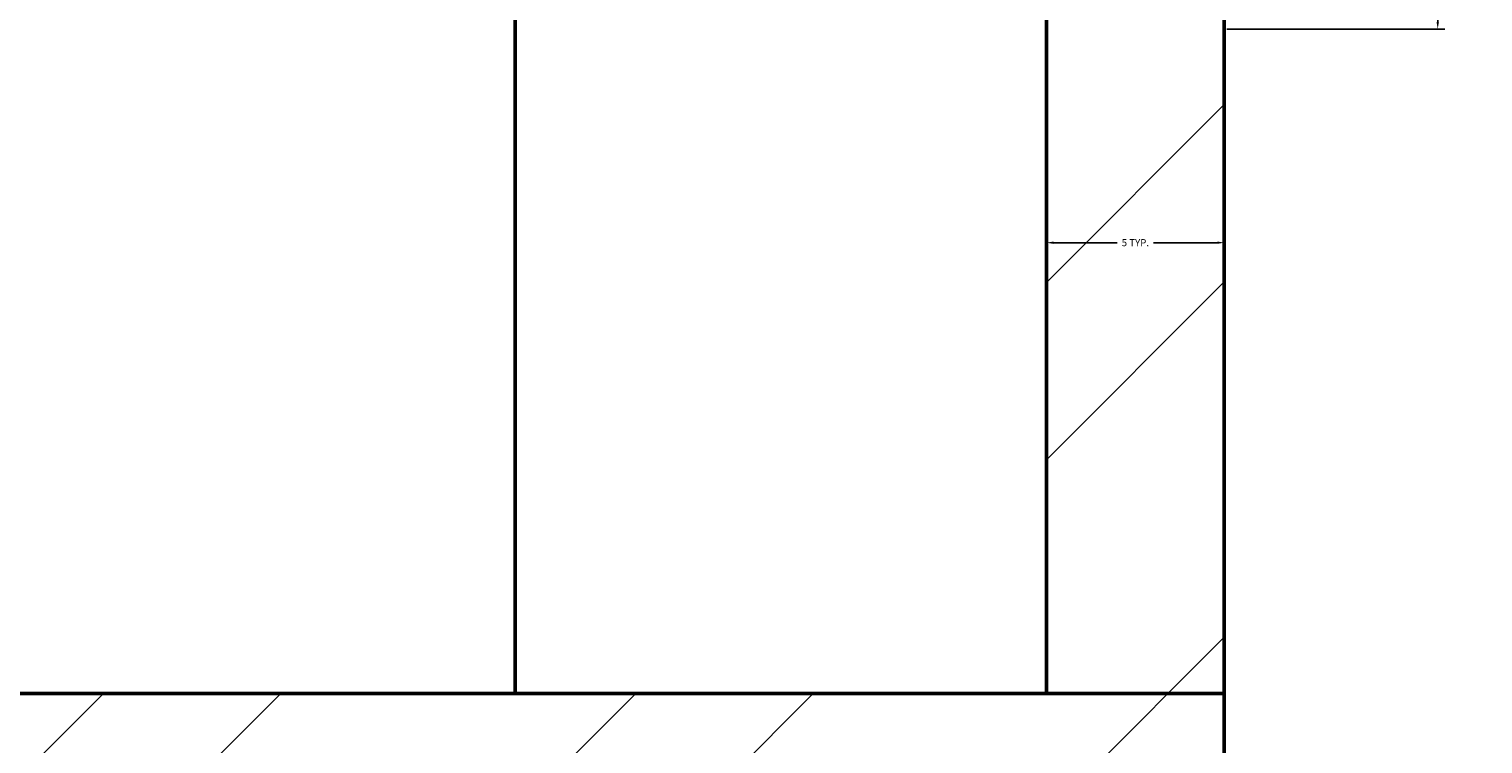
# Model space of a CAD drawing. Units: inches. Extents: x 1901 to 2863, y 888 to 2433.
# Tile 86 of 91: x 2723 to 2759, y 2009 to 2027. Entities that reach past the tile are written whole.
import ezdxf

# ---------------------------------------------------------------- set-up
doc = ezdxf.new("R2010")
doc.units = ezdxf.units.IN
for name, color, linetype, lineweight in [('A-ANNO-DIMS', 2, 'Continuous', 18), ('A-WALL', 7, 'Continuous', 50), ('A-WALL-PATT', 8, 'Continuous', 13)]:
    doc.layers.add(name, color=color, linetype=linetype, lineweight=lineweight)
doc.styles.get("Standard").update_dxf_attribs({"font": 'arial.ttf'})
doc.dimstyles.get("Standard").update_dxf_attribs({"dimtxt": 0.18, "dimasz": 0.18, "dimexe": 0.18, "dimexo": 0.0625, "dimgap": 0.09, "dimtad": 0, "dimtih": 1, "dimtoh": 1, "dimdec": 4, "dimzin": 0, "dimdsep": 46, "dimtxsty": 'Standard', "dimcen": 0.09, "dimadec": 0, "dimazin": 0, "dimtfac": 1, "dimtdec": 4, "dimtofl": 0, "dimtmove": 0, "dimatfit": 3, "dimfxl": 1, "dimtolj": 1, "dimtzin": 0, "dimarcsym": 0})

# ---------------------------------------------------------------- blocks, each defined once
blk = doc.blocks.new('*D29')
at = {"layer": 'A-ANNO-DIMS', "color": 0, "lineweight": -2, "transparency": 16777216}
for p, q in [((2752.989, 2063.429), (2758.506, 2063.429)), ((2758.326, 2063.249), (2758.326, 2045.612)), ((2758.326, 2027.609), (2758.326, 2045.245)), ((2752.989, 2027.429), (2758.506, 2027.429))]:
    blk.add_line(p, q, dxfattribs=at)
at = {"layer": 'A-ANNO-DIMS', "color": 0, "transparency": 16777216}
for points in [[(2758.296, 2063.249), (2758.356, 2063.249), (2758.326, 2063.429)], [(2758.296, 2027.609), (2758.356, 2027.609), (2758.326, 2027.429)]]:
    blk.add_solid(points, dxfattribs=at)
at = {"layer": 'Defpoints', "color": 0, "transparency": 16777216}
for p in [(2752.926, 2063.429), (2758.326, 2063.429), (2752.926, 2027.429)]:
    blk.add_point(p, dxfattribs=at)
at = {"layer": 'A-ANNO-DIMS', "color": 0, "transparency": 16777216, "insert": (2758.326, 2045.429), "char_height": 0.18, "attachment_point": 5}
blk.add_mtext('\\A1;WINDOW W6 36 TYP.', dxfattribs=at)
blk = doc.blocks.new('*D30')
at = {"layer": 'A-ANNO-DIMS', "color": 0, "lineweight": -2, "transparency": 16777216}
for p, q in [((2748.426, 2027.366), (2748.426, 2021.849)), ((2752.926, 2027.366), (2752.926, 2021.849)), ((2748.606, 2022.029), (2750.218, 2022.029)), ((2752.746, 2022.029), (2751.134, 2022.029))]:
    blk.add_line(p, q, dxfattribs=at)
at = {"layer": 'A-ANNO-DIMS', "color": 0, "transparency": 16777216}
for points in [[(2748.606, 2022.059), (2748.606, 2021.999), (2748.426, 2022.029)], [(2752.746, 2022.059), (2752.746, 2021.999), (2752.926, 2022.029)]]:
    blk.add_solid(points, dxfattribs=at)
at = {"layer": 'Defpoints', "color": 0, "transparency": 16777216}
for p in [(2748.426, 2027.429), (2752.926, 2027.429), (2752.926, 2022.029)]:
    blk.add_point(p, dxfattribs=at)
at = {"layer": 'A-ANNO-DIMS', "color": 0, "transparency": 16777216, "insert": (2750.676, 2022.029), "char_height": 0.18, "attachment_point": 5}
blk.add_mtext('\\A1;5 TYP.', dxfattribs=at)

msp = doc.modelspace()

# ---------------------------------------------------------------- hatches: boundary and pattern name
at = {"layer": 'A-WALL-PATT'}
h = msp.add_hatch(dxfattribs=at)
h.set_pattern_fill('ANSI32', color=256)
h.paths.add_polyline_path([(2192.501, 2274.134), (2141.264, 2274.134), (2141.264, 2269.634), (2192.501, 2269.634)])
h.paths.add_polyline_path([(2259.926, 2274.134), (2216.501, 2274.134), (2216.501, 2269.634), (2255.426, 2269.634), (2255.426, 2214.634), (2250.809, 2214.634), (2250.809, 2210.134), (2259.926, 2210.134), (2259.926, 2215.134), (2271.756, 2215.134), (2271.756, 2217.384), (2271.756, 2219.634), (2259.926, 2219.634)])
h.paths.add_polyline_path([(2171.426, 2269.634), (2166.926, 2269.634), (2166.926, 2219.634), (2121.238, 2219.634), (2121.238, 2215.134), (2166.926, 2215.134), (2166.926, 2083.134), (2161.807, 2083.134), (2161.807, 2078.634), (2171.426, 2078.634), (2176.996, 2078.634), (2176.996, 2080.884), (2176.996, 2083.134), (2171.426, 2083.134), (2171.426, 2210.134), (2230.912, 2210.134), (2230.912, 2212.384), (2230.912, 2214.634), (2171.426, 2214.634)])
h.paths.add_polyline_path([(2117.264, 2274.134), (2089.426, 2274.134), (2089.426, 2219.634), (2081.136, 2219.634), (2081.136, 2215.134), (2089.426, 2215.134), (2098.004, 2215.134), (2098.004, 2217.384), (2098.004, 2219.634), (2093.926, 2219.634), (2093.926, 2269.634), (2117.264, 2269.634), (2117.264, 2271.884)])
h.paths.add_polyline_path([(2343.426, 2219.634), (2329.295, 2219.634), (2329.295, 2215.134), (2338.926, 2215.134), (2338.926, 2184.739), (2343.426, 2184.739)])
h.paths.add_polyline_path([(2338.926, 2083.134), (2329.295, 2083.134), (2208.966, 2083.134), (2208.966, 2078.634), (2338.926, 2078.634)])
h.paths.add_polyline_path([(2343.426, 2136.739), (2338.926, 2136.739), (2338.926, 1872.634), (2343.426, 1872.634)])
h.paths.add_polyline_path([(2343.426, 1863.634), (2397.68, 1863.634), (2397.68, 1821.634), (2384.138, 1821.634), (2384.138, 1812.634), (2418.33, 1812.634), (2418.33, 1817.134), (2418.33, 1821.634), (2406.68, 1821.634), (2406.68, 1863.634), (2459.499, 1863.634), (2459.499, 1821.634), (2447.138, 1821.634), (2447.138, 1812.634), (2459.499, 1812.634), (2468.499, 1812.634), (2468.499, 1872.634), (2394.426, 1872.634), (2334.426, 1872.634), (2334.426, 1812.634), (2343.426, 1812.634), (2353.251, 1812.634), (2353.251, 1821.634), (2343.426, 1821.634)])
h.paths.add_polyline_path([(2510.014, 1872.634), (2468.499, 1872.634), (2468.499, 1868.134), (2510.014, 1868.134)])
h.paths.add_polyline_path([(2514.009, 1817.134), (2468.499, 1817.134), (2468.499, 1812.634), (2482.114, 1812.634), (2482.114, 1800.606), (2486.614, 1800.606), (2486.614, 1812.634), (2514.009, 1812.634)])
h.paths.add_polyline_path([(2299.247, 1814.884), (2299.247, 1817.134), (2295.926, 1817.134), (2295.926, 1854.169), (2293.676, 1854.169), (2291.426, 1854.169), (2291.426, 1817.134), (2266.109, 1817.134), (2266.109, 1812.634), (2299.247, 1812.634)])
h.paths.add_polyline_path([(2218.109, 1817.134), (2206.46, 1817.134), (2171.426, 1817.134), (2171.426, 1949.134), (2190.1, 1949.134), (2190.1, 1953.634), (2163.468, 1953.634), (2163.468, 1949.134), (2166.926, 1949.134), (2166.926, 1817.134), (2114.297, 1817.134), (2114.297, 1812.634), (2218.109, 1812.634)])
h.paths.add_polyline_path([(2029.426, 1970.922), (2024.926, 1970.922), (2024.926, 1912.717), (2029.426, 1912.717)])
h.paths.add_polyline_path([(2132.297, 1953.634), (2113.926, 1953.634), (2113.926, 1975.888), (2111.676, 1975.888), (2109.426, 1975.888), (2109.426, 1953.634), (2029.426, 1953.634), (2029.426, 1949.134), (2132.297, 1949.134)])
h.paths.add_polyline_path([(2029.426, 1853.606), (2029.31, 1853.606), (2029.31, 1853.606), (2029.426, 1853.606), (2029.426, 1864.717), (2024.926, 1864.717), (2024.926, 1812.634), (2066.297, 1812.634), (2066.297, 1814.884), (2066.297, 1817.134), (2029.426, 1817.134)])
h.paths.add_polyline_path([(2122.926, 2010.088), (2120.676, 2010.088), (2118.426, 2010.088), (2118.426, 2006.134), (2029.426, 2006.134), (2029.426, 2001.634), (2109.426, 2001.634), (2109.426, 1998.041), (2113.926, 1998.041), (2113.926, 2001.634), (2122.926, 2001.634)])
h.paths.add_polyline_path([(2029.426, 2031.376), (2024.926, 2031.376), (2024.926, 1994.922), (2027.176, 1994.922), (2029.426, 1994.922)])
h.paths.add_polyline_path([(2029.426, 2136.739), (2024.926, 2136.739), (2024.926, 2067.376), (2027.176, 2067.376), (2029.426, 2067.376)])
h.paths.add_polyline_path([(2125.618, 2083.134), (2029.426, 2083.134), (2029.426, 2078.634), (2118.426, 2078.634), (2118.426, 2030.715), (2122.926, 2030.715), (2122.926, 2078.634), (2125.618, 2078.634)])
h.paths.add_polyline_path([(2029.426, 2215.134), (2040.468, 2215.134), (2040.468, 2217.384), (2040.468, 2219.634), (2024.926, 2219.634), (2024.926, 2184.739), (2029.426, 2184.739), (2029.426, 2187.778)])
h.paths.add_polyline_path([(2686.426, 2274.134), (2659.284, 2274.134), (2659.284, 2269.634), (2681.926, 2269.634), (2681.926, 2219.634), (2676.816, 2219.634), (2676.816, 2215.134), (2681.926, 2215.134), (2697.011, 2215.134), (2697.011, 2217.384), (2697.011, 2219.634), (2686.426, 2219.634)])
h.paths.add_polyline_path([(2609.926, 2269.634), (2635.284, 2269.634), (2635.284, 2274.134), (2571.431, 2274.134), (2571.431, 2269.634), (2605.426, 2269.634), (2605.426, 2214.634), (2549.098, 2214.634), (2549.098, 2210.134), (2605.426, 2210.134), (2605.426, 2083.134), (2601.014, 2083.134), (2601.014, 2080.884), (2601.014, 2078.634), (2609.926, 2078.634), (2616.162, 2078.634), (2616.162, 2080.884), (2616.162, 2083.134), (2609.926, 2083.134), (2609.926, 2215.134), (2651.465, 2215.134), (2651.465, 2217.384), (2651.465, 2219.634), (2609.926, 2219.634)])
h.paths.add_polyline_path([(2521.426, 2269.634), (2547.431, 2269.634), (2547.431, 2271.884), (2547.431, 2274.134), (2516.926, 2274.134), (2516.926, 2219.634), (2506.41, 2219.634), (2506.41, 2215.134), (2516.926, 2215.134), (2516.926, 2210.134), (2525.402, 2210.134), (2525.402, 2212.384), (2525.402, 2214.634), (2521.426, 2214.634)])
h.paths.add_polyline_path([(2456.011, 2219.634), (2439.426, 2219.634), (2439.426, 2187.888), (2443.926, 2187.888), (2443.926, 2215.134), (2456.011, 2215.134)])
h.paths.add_polyline_path([(2752.926, 2219.634), (2739.485, 2219.634), (2739.485, 2215.134), (2748.426, 2215.134), (2748.426, 2187.888), (2752.926, 2187.888)])
h.paths.add_polyline_path([(2752.926, 2139.888), (2748.426, 2139.888), (2748.426, 2083.134), (2648.416, 2083.134), (2648.416, 2078.634), (2654.926, 2078.634), (2654.926, 2039.437), (2659.426, 2039.437), (2659.426, 2078.634), (2748.426, 2078.634), (2748.426, 2063.429), (2752.926, 2063.429)])
h.paths.add_polyline_path([(2752.926, 2010.634), (2659.426, 2010.634), (2659.426, 2015.652), (2654.926, 2015.652), (2654.926, 2010.634), (2605.426, 2010.634), (2605.426, 1920.967), (2609.926, 1920.967), (2609.926, 2006.134), (2748.426, 2006.134), (2748.426, 1982.466), (2752.926, 1982.466)])
h.paths.add_polyline_path([(2752.926, 2027.429), (2748.426, 2027.429), (2748.426, 2010.634), (2752.926, 2010.634)])
h.paths.add_polyline_path([(2748.426, 1886.134), (2609.926, 1886.134), (2609.926, 1889.719), (2605.426, 1889.719), (2605.426, 1861.262), (2609.926, 1861.262), (2609.926, 1881.634), (2748.426, 1881.634)])
h.paths.add_polyline_path([(2456.855, 2228.831), (2498.401, 2228.831), (2498.401, 2247.488), (2456.855, 2247.488)], flags=9)
h.paths.add_polyline_path([(2038.602, 2237.418), (2080.174, 2237.418), (2080.174, 2256.075), (2038.602, 2256.075)], flags=9)
h.paths.add_polyline_path([(2292.009, 1062.394), (2539.932, 1062.394), (2539.932, 1099.487), (2292.009, 1099.487)], flags=9)
h.paths.add_polyline_path([(2424.91, 1832.253), (2448.513, 1832.253), (2448.513, 1846.678), (2424.91, 1846.678)], flags=25)
h.paths.add_polyline_path([(2359.076, 1832.253), (2382.678, 1832.253), (2382.678, 1846.678), (2359.076, 1846.678)], flags=25)
h.paths.add_polyline_path([(2352.899, 1684.802), (2367.543, 1684.802), (2367.543, 1697.167), (2352.899, 1697.167)], flags=9)
h.paths.add_polyline_path([(2079.288, 1755.826), (2169.024, 1755.826), (2169.024, 1774.372), (2079.288, 1774.372)], flags=9)
h.paths.add_polyline_path([(2404.09, 1373.857), (2404.09, 1463.593), (2385.544, 1463.593), (2385.544, 1373.857)], flags=9)
h.paths.add_polyline_path([(2268.091, 2236.371), (2309.636, 2236.371), (2309.636, 2255.028), (2268.091, 2255.028)], flags=9)
h.paths.add_polyline_path([(2575.96, 1700.951), (2665.696, 1700.951), (2665.696, 1719.498), (2575.96, 1719.498)], flags=9)
h.paths.add_polyline_path([(2302.962, 1878.474), (2329.524, 1878.474), (2329.524, 1888.777), (2302.962, 1888.777)], flags=9)
h.paths.add_polyline_path([(2097.415, 2240.576), (2126.573, 2240.576), (2126.573, 2259.233), (2097.415, 2259.233)], flags=9)
h.paths.add_polyline_path([(2208.725, 2246.124), (2237.882, 2246.124), (2237.882, 2264.781), (2208.725, 2264.781)], flags=9)
h.paths.add_polyline_path([(2038.147, 1925.958), (2076.987, 1925.958), (2076.987, 1944.615), (2038.147, 1944.615)], flags=9)
h.paths.add_polyline_path([(2239.144, 1926.672), (2288.465, 1926.672), (2288.465, 1945.329), (2239.144, 1945.329)], flags=9)
h.paths.add_polyline_path([(2175.429, 2007.33), (2212.356, 2007.33), (2212.356, 2025.987), (2175.429, 2025.987)], flags=9)
h.paths.add_polyline_path([(2225.034, 2091.794), (2263.875, 2091.794), (2263.875, 2110.451), (2225.034, 2110.451)], flags=9)
h.paths.add_polyline_path([(2035.398, 2098.478), (2074.238, 2098.478), (2074.238, 2117.135), (2035.398, 2117.135)], flags=9)
h.paths.add_polyline_path([(2050.102, 2029.209), (2083.26, 2029.209), (2083.26, 2047.866), (2050.102, 2047.866)], flags=9)
h.paths.add_polyline_path([(2069.677, 1956.719), (2098.835, 1956.719), (2098.835, 1975.376), (2069.677, 1975.376)], flags=25)
h.paths.add_polyline_path([(2328.62, 1753.336), (2361.663, 1753.336), (2361.663, 1771.993), (2328.62, 1771.993)], flags=9)
h.paths.add_polyline_path([(2395.162, 2060.888), (2395.162, 2140.654), (2378.676, 2140.654), (2378.676, 2060.888)], flags=9)
h.paths.add_polyline_path([(2463.728, 2059.02), (2492.886, 2059.02), (2492.886, 2077.677), (2463.728, 2077.677)], flags=9)
h.paths.add_polyline_path([(2458.027, 2181.536), (2496.868, 2181.536), (2496.868, 2200.194), (2458.027, 2200.194)], flags=9)
h.paths.add_polyline_path([(2527.577, 2243.074), (2556.735, 2243.074), (2556.735, 2261.731), (2527.577, 2261.731)], flags=9)
h.paths.add_polyline_path([(2694.461, 2232.767), (2736.033, 2232.767), (2736.033, 2251.425), (2694.461, 2251.425)], flags=9)
h.paths.add_polyline_path([(2637.821, 2249.225), (2666.979, 2249.225), (2666.979, 2267.882), (2637.821, 2267.882)], flags=9)
h.paths.add_polyline_path([(2623.687, 2183.541), (2662.528, 2183.541), (2662.528, 2202.199), (2623.687, 2202.199)], flags=9)
h.paths.add_polyline_path([(2691.965, 2021.5), (2725.124, 2021.5), (2725.124, 2040.157), (2691.965, 2040.157)], flags=9)
h.paths.add_polyline_path([(2621.043, 1975.912), (2662.335, 1975.912), (2662.335, 1994.569), (2621.043, 1994.569)], flags=25)
h.paths.add_polyline_path([(2479.032, 1927.62), (2519.844, 1927.62), (2519.844, 1946.277), (2479.032, 1946.277)], flags=9)
h.paths.add_polyline_path([(2670.941, 1849.076), (2716.005, 1849.076), (2716.005, 1867.734), (2670.941, 1867.734)], flags=9)
h.paths.add_polyline_path([(2523.613, 1782.956), (2550.175, 1782.956), (2550.175, 1793.26), (2523.613, 1793.26)], flags=9)
h.paths.add_polyline_path([(2450.841, 1207.331), (2492.386, 1207.331), (2492.386, 1225.989), (2450.841, 1225.989)], flags=9)
h.paths.add_polyline_path([(2527.751, 1203.841), (2556.908, 1203.841), (2556.908, 1222.499), (2527.751, 1222.499)], flags=9)
h.paths.add_polyline_path([(2639.111, 1207.2), (2668.268, 1207.2), (2668.268, 1225.857), (2639.111, 1225.857)], flags=9)
h.paths.add_polyline_path([(2692.594, 1218.965), (2734.167, 1218.965), (2734.167, 1237.623), (2692.594, 1237.623)], flags=9)
h.paths.add_polyline_path([(2669.266, 1366.329), (2708.106, 1366.329), (2708.106, 1384.987), (2669.266, 1384.987)], flags=9)
h.paths.add_polyline_path([(2463.313, 1358.031), (2502.153, 1358.031), (2502.153, 1376.688), (2463.313, 1376.688)], flags=9)
h.paths.add_polyline_path([(2494.725, 1449.963), (2531.652, 1449.963), (2531.652, 1468.62), (2494.725, 1468.62)], flags=9)
h.paths.add_polyline_path([(2675.565, 1422.157), (2708.724, 1422.157), (2708.724, 1440.815), (2675.565, 1440.815)], flags=9)
h.paths.add_polyline_path([(2685.634, 1493.891), (2714.792, 1493.891), (2714.792, 1512.548), (2685.634, 1512.548)], flags=9)
h.paths.add_polyline_path([(2686.805, 1529.913), (2725.645, 1529.913), (2725.645, 1548.57), (2686.805, 1548.57)], flags=9)
h.paths.add_polyline_path([(2503.651, 1537.991), (2552.972, 1537.991), (2552.972, 1556.648), (2503.651, 1556.648)], flags=9)
h.paths.add_polyline_path([(2291.713, 1643.504), (2318.275, 1643.504), (2318.275, 1653.807), (2291.713, 1653.807)], flags=9)
h.paths.add_polyline_path([(2450.626, 1610.52), (2477.189, 1610.52), (2477.189, 1620.824), (2450.626, 1620.824)], flags=9)
h.paths.add_polyline_path([(2359.985, 1551.814), (2422.253, 1551.814), (2422.253, 1562.117), (2359.985, 1562.117)], flags=9)
h.paths.add_polyline_path([(2280.106, 1249.006), (2321.651, 1249.006), (2321.651, 1267.663), (2280.106, 1267.663)], flags=9)
h.paths.add_polyline_path([(2164.057, 1274.232), (2193.215, 1274.232), (2193.215, 1292.889), (2164.057, 1292.889)], flags=9)
h.paths.add_polyline_path([(2118.21, 1277.694), (2151.252, 1277.694), (2151.252, 1296.351), (2118.21, 1296.351)], flags=9)
h.paths.add_polyline_path([(2031.946, 1268.529), (2073.519, 1268.529), (2073.519, 1287.187), (2031.946, 1287.187)], flags=9)
h.paths.add_polyline_path([(2050.199, 1409.079), (2089.04, 1409.079), (2089.04, 1427.736), (2050.199, 1427.736)], flags=9)
h.paths.add_polyline_path([(2243.743, 1421.032), (2282.584, 1421.032), (2282.584, 1439.689), (2243.743, 1439.689)], flags=9)
h.paths.add_polyline_path([(2190.746, 1509.769), (2231.558, 1509.769), (2231.558, 1528.426), (2190.746, 1528.426)], flags=9)
h.paths.add_polyline_path([(2058.392, 1475.415), (2091.55, 1475.415), (2091.55, 1494.073), (2058.392, 1494.073)], flags=9)
h.paths.add_polyline_path([(2062.447, 1553.09), (2091.605, 1553.09), (2091.605, 1571.747), (2062.447, 1571.747)], flags=9)
h.paths.add_polyline_path([(2219.524, 1590.365), (2266.147, 1590.365), (2266.147, 1609.022), (2219.524, 1609.022)], flags=9)
h.paths.add_polyline_path([(2041.072, 1584.188), (2079.912, 1584.188), (2079.912, 1602.845), (2041.072, 1602.845)], flags=9)
h = msp.add_hatch(dxfattribs=at)
h.set_pattern_fill('ANSI32', color=256)
h.paths.add_polyline_path([(2443.926, 2139.888), (2439.426, 2139.888), (2439.426, 2069.348), (2441.676, 2069.348), (2443.926, 2069.348), (2443.926, 2078.634), (2521.926, 2078.634), (2521.926, 2075.067), (2524.176, 2075.067), (2526.426, 2075.067), (2526.426, 2078.634), (2571.755, 2078.634), (2571.755, 2080.884), (2571.755, 2083.134), (2443.926, 2083.134)])
h.paths.add_polyline_path([(2526.426, 2054.634), (2524.176, 2054.634), (2521.926, 2054.634), (2521.926, 2030.634), (2443.926, 2030.634), (2443.926, 2045.348), (2439.426, 2045.348), (2439.426, 1983.867), (2443.926, 1983.867), (2443.926, 2026.134), (2521.926, 2026.134), (2526.426, 2026.134)])
h.paths.add_polyline_path([(2443.926, 1923.867), (2439.426, 1923.867), (2439.426, 1872.634), (2443.926, 1872.634)])
h.paths.add_polyline_path([(2636.233, 1766.134), (2609.926, 1766.134), (2609.926, 1779.785), (2605.426, 1779.785), (2605.426, 1766.134), (2486.614, 1766.134), (2486.614, 1770.671), (2482.114, 1770.671), (2482.114, 1766.134), (2482.114, 1761.634), (2636.233, 1761.634), (2636.233, 1763.884)])
h.paths.add_polyline_path([(2519.536, 1663.384), (2519.536, 1665.634), (2494.926, 1665.634), (2481.831, 1665.634), (2481.831, 1663.384), (2481.831, 1661.134), (2490.426, 1661.134), (2490.426, 1640.157), (2494.926, 1640.157), (2494.926, 1661.134), (2519.536, 1661.134)])
h.paths.add_polyline_path([(2443.926, 1712.134), (2443.926, 1716.634), (2414.464, 1716.634), (2414.464, 1712.134), (2439.426, 1712.134), (2439.426, 1545.507), (2443.926, 1545.507), (2443.926, 1661.134), (2448.475, 1661.134), (2448.475, 1665.634), (2443.926, 1665.634)])
h.paths.add_polyline_path([(2343.426, 1712.134), (2365.525, 1712.134), (2365.525, 1714.384), (2365.525, 1716.634), (2333.871, 1716.634), (2333.871, 1714.384), (2333.871, 1712.134), (2338.926, 1712.134), (2338.926, 1575.634), (2338.926, 1545.507), (2343.426, 1545.507), (2343.426, 1547.507), (2343.426, 1580.134)])
h.paths.add_polyline_path([(2752.926, 1665.634), (2579.536, 1665.634), (2579.536, 1661.134), (2615.926, 1661.134), (2615.926, 1529.134), (2598.931, 1529.134), (2598.931, 1524.634), (2623.127, 1524.634), (2623.127, 1526.884), (2623.127, 1529.134), (2620.426, 1529.134), (2620.426, 1661.134), (2748.426, 1661.134), (2748.426, 1633.499), (2752.926, 1633.499)])
h.paths.add_polyline_path([(2752.926, 1419.929), (2748.426, 1419.929), (2748.426, 1400.134), (2659.426, 1400.134), (2659.426, 1444.333), (2657.176, 1444.333), (2654.926, 1444.333), (2654.926, 1400.134), (2643.649, 1400.134), (2643.649, 1395.634), (2748.426, 1395.634), (2748.426, 1364.035), (2752.926, 1364.035)])
h.paths.add_polyline_path([(2752.926, 1492.878), (2748.426, 1492.878), (2748.426, 1476.634), (2667.426, 1476.634), (2667.426, 1479.71), (2665.176, 1479.71), (2662.926, 1479.71), (2662.926, 1476.634), (2654.926, 1476.634), (2654.926, 1469.536), (2659.426, 1469.536), (2659.426, 1472.134), (2748.426, 1472.134), (2748.426, 1455.929), (2752.926, 1455.929)])
h.paths.add_polyline_path([(2752.926, 1304.035), (2748.426, 1304.035), (2748.426, 1263.634), (2738.66, 1263.634), (2738.66, 1259.134), (2752.926, 1259.134)])
h.paths.add_polyline_path([(2685.926, 1259.134), (2695.49, 1259.134), (2695.49, 1261.384), (2695.49, 1263.634), (2677.837, 1263.634), (2677.837, 1261.384), (2677.837, 1259.134), (2681.426, 1259.134), (2681.426, 1203.634), (2653.277, 1203.634), (2653.277, 1199.134), (2685.926, 1199.134), (2685.926, 1203.634)])
h.paths.add_polyline_path([(2609.426, 1395.634), (2611.848, 1395.634), (2611.848, 1400.134), (2598.888, 1400.134), (2598.888, 1397.884), (2598.888, 1395.634), (2604.926, 1395.634), (2604.926, 1268.134), (2554.726, 1268.134), (2554.726, 1265.884), (2554.726, 1263.634), (2604.926, 1263.634), (2604.926, 1203.634), (2571.306, 1203.634), (2571.306, 1199.134), (2604.926, 1199.134), (2629.277, 1199.134), (2629.277, 1201.384), (2629.277, 1203.634), (2609.426, 1203.634), (2609.426, 1258.634), (2609.426, 1259.134), (2654.804, 1259.134), (2654.804, 1263.634), (2609.426, 1263.634)])
h.paths.add_polyline_path([(2443.926, 1304.035), (2439.426, 1304.035), (2439.426, 1259.134), (2443.926, 1259.134), (2456.16, 1259.134), (2456.16, 1261.384), (2456.16, 1263.634), (2443.926, 1263.634)])
h.paths.add_polyline_path([(2525.426, 1263.634), (2531.778, 1263.634), (2531.778, 1268.134), (2520.926, 1268.134), (2520.926, 1263.634), (2511.409, 1263.634), (2511.409, 1259.134), (2520.926, 1259.134), (2520.926, 1199.134), (2547.306, 1199.134), (2547.306, 1201.384), (2547.306, 1203.634), (2525.426, 1203.634)])
h.paths.add_polyline_path([(2443.926, 1434.842), (2439.426, 1434.842), (2439.426, 1364.035), (2441.676, 1364.035), (2443.926, 1364.035)])
h.paths.add_polyline_path([(2567.134, 1400.134), (2443.926, 1400.134), (2443.926, 1395.634), (2567.134, 1395.634)])
h.paths.add_polyline_path([(2443.926, 1545.507), (2439.426, 1545.507), (2439.426, 1494.842), (2443.926, 1494.842)])
h.paths.add_polyline_path([(2494.926, 1553.349), (2492.676, 1553.349), (2490.426, 1553.349), (2490.426, 1524.634), (2494.926, 1524.634), (2525.936, 1524.634), (2525.936, 1526.884), (2525.936, 1529.134), (2494.926, 1529.134)])
h.paths.add_polyline_path([(2752.926, 1573.499), (2748.426, 1573.499), (2748.426, 1529.134), (2657.759, 1529.134), (2657.759, 1524.634), (2662.926, 1524.634), (2662.926, 1498.631), (2667.426, 1498.631), (2667.426, 1524.634), (2748.426, 1524.634), (2748.426, 1516.878), (2752.926, 1516.878)])
h.paths.add_polyline_path([(2038.602, 2237.418), (2080.174, 2237.418), (2080.174, 2256.075), (2038.602, 2256.075)], flags=9)
h.paths.add_polyline_path([(2292.009, 1062.394), (2539.932, 1062.394), (2539.932, 1099.487), (2292.009, 1099.487)], flags=9)
h.paths.add_polyline_path([(2424.91, 1832.253), (2448.513, 1832.253), (2448.513, 1846.678), (2424.91, 1846.678)], flags=9)
h.paths.add_polyline_path([(2359.076, 1832.253), (2382.678, 1832.253), (2382.678, 1846.678), (2359.076, 1846.678)], flags=9)
h.paths.add_polyline_path([(2352.899, 1684.802), (2367.543, 1684.802), (2367.543, 1697.167), (2352.899, 1697.167)], flags=9)
h.paths.add_polyline_path([(2079.288, 1755.826), (2169.024, 1755.826), (2169.024, 1774.372), (2079.288, 1774.372)], flags=9)
h.paths.add_polyline_path([(2404.09, 1373.857), (2404.09, 1463.593), (2385.544, 1463.593), (2385.544, 1373.857)], flags=9)
h.paths.add_polyline_path([(2268.091, 2236.371), (2309.636, 2236.371), (2309.636, 2255.028), (2268.091, 2255.028)], flags=9)
h.paths.add_polyline_path([(2575.96, 1700.951), (2665.696, 1700.951), (2665.696, 1719.498), (2575.96, 1719.498)], flags=9)
h.paths.add_polyline_path([(2302.962, 1878.474), (2329.524, 1878.474), (2329.524, 1888.777), (2302.962, 1888.777)], flags=9)
h.paths.add_polyline_path([(2097.415, 2240.576), (2126.573, 2240.576), (2126.573, 2259.233), (2097.415, 2259.233)], flags=9)
h.paths.add_polyline_path([(2208.725, 2246.124), (2237.882, 2246.124), (2237.882, 2264.781), (2208.725, 2264.781)], flags=9)
h.paths.add_polyline_path([(2038.147, 1925.958), (2076.987, 1925.958), (2076.987, 1944.615), (2038.147, 1944.615)], flags=9)
h.paths.add_polyline_path([(2239.144, 1926.672), (2288.465, 1926.672), (2288.465, 1945.329), (2239.144, 1945.329)], flags=9)
h.paths.add_polyline_path([(2175.429, 2007.33), (2212.356, 2007.33), (2212.356, 2025.987), (2175.429, 2025.987)], flags=9)
h.paths.add_polyline_path([(2225.034, 2091.794), (2263.875, 2091.794), (2263.875, 2110.451), (2225.034, 2110.451)], flags=9)
h.paths.add_polyline_path([(2035.398, 2098.478), (2074.238, 2098.478), (2074.238, 2117.135), (2035.398, 2117.135)], flags=9)
h.paths.add_polyline_path([(2050.102, 2029.209), (2083.26, 2029.209), (2083.26, 2047.866), (2050.102, 2047.866)], flags=9)
h.paths.add_polyline_path([(2069.677, 1956.719), (2098.835, 1956.719), (2098.835, 1975.376), (2069.677, 1975.376)], flags=9)
h.paths.add_polyline_path([(2328.62, 1753.336), (2361.663, 1753.336), (2361.663, 1771.993), (2328.62, 1771.993)], flags=9)
h.paths.add_polyline_path([(2395.162, 2060.888), (2395.162, 2140.654), (2378.676, 2140.654), (2378.676, 2060.888)], flags=9)
h.paths.add_polyline_path([(2463.728, 2059.02), (2492.886, 2059.02), (2492.886, 2077.677), (2463.728, 2077.677)], flags=9)
h.paths.add_polyline_path([(2458.027, 2181.536), (2496.868, 2181.536), (2496.868, 2200.194), (2458.027, 2200.194)], flags=9)
h.paths.add_polyline_path([(2456.855, 2228.831), (2498.401, 2228.831), (2498.401, 2247.488), (2456.855, 2247.488)], flags=9)
h.paths.add_polyline_path([(2527.577, 2243.074), (2556.735, 2243.074), (2556.735, 2261.731), (2527.577, 2261.731)], flags=9)
h.paths.add_polyline_path([(2694.461, 2232.767), (2736.033, 2232.767), (2736.033, 2251.425), (2694.461, 2251.425)], flags=9)
h.paths.add_polyline_path([(2637.821, 2249.225), (2666.979, 2249.225), (2666.979, 2267.882), (2637.821, 2267.882)], flags=9)
h.paths.add_polyline_path([(2623.687, 2183.541), (2662.528, 2183.541), (2662.528, 2202.199), (2623.687, 2202.199)], flags=9)
h.paths.add_polyline_path([(2691.965, 2021.5), (2725.124, 2021.5), (2725.124, 2040.157), (2691.965, 2040.157)], flags=9)
h.paths.add_polyline_path([(2621.043, 1975.912), (2662.335, 1975.912), (2662.335, 1994.569), (2621.043, 1994.569)], flags=9)
h.paths.add_polyline_path([(2479.032, 1927.62), (2519.844, 1927.62), (2519.844, 1946.277), (2479.032, 1946.277)], flags=9)
h.paths.add_polyline_path([(2670.941, 1849.076), (2716.005, 1849.076), (2716.005, 1867.734), (2670.941, 1867.734)], flags=9)
h.paths.add_polyline_path([(2523.613, 1782.956), (2550.175, 1782.956), (2550.175, 1793.26), (2523.613, 1793.26)], flags=9)
h.paths.add_polyline_path([(2450.841, 1207.331), (2492.386, 1207.331), (2492.386, 1225.989), (2450.841, 1225.989)], flags=9)
h.paths.add_polyline_path([(2527.751, 1203.841), (2556.908, 1203.841), (2556.908, 1222.499), (2527.751, 1222.499)], flags=9)
h.paths.add_polyline_path([(2639.111, 1207.2), (2668.268, 1207.2), (2668.268, 1225.857), (2639.111, 1225.857)], flags=9)
h.paths.add_polyline_path([(2692.594, 1218.965), (2734.167, 1218.965), (2734.167, 1237.623), (2692.594, 1237.623)], flags=9)
h.paths.add_polyline_path([(2669.266, 1366.329), (2708.106, 1366.329), (2708.106, 1384.987), (2669.266, 1384.987)], flags=25)
h.paths.add_polyline_path([(2463.313, 1358.031), (2502.153, 1358.031), (2502.153, 1376.688), (2463.313, 1376.688)], flags=9)
h.paths.add_polyline_path([(2494.725, 1449.963), (2531.652, 1449.963), (2531.652, 1468.62), (2494.725, 1468.62)], flags=9)
h.paths.add_polyline_path([(2675.565, 1422.157), (2708.724, 1422.157), (2708.724, 1440.815), (2675.565, 1440.815)], flags=25)
h.paths.add_polyline_path([(2685.634, 1493.891), (2714.792, 1493.891), (2714.792, 1512.548), (2685.634, 1512.548)], flags=9)
h.paths.add_polyline_path([(2686.805, 1529.913), (2725.645, 1529.913), (2725.645, 1548.57), (2686.805, 1548.57)], flags=25)
h.paths.add_polyline_path([(2503.651, 1537.991), (2552.972, 1537.991), (2552.972, 1556.648), (2503.651, 1556.648)], flags=9)
h.paths.add_polyline_path([(2291.713, 1643.504), (2318.275, 1643.504), (2318.275, 1653.807), (2291.713, 1653.807)], flags=9)
h.paths.add_polyline_path([(2450.626, 1610.52), (2477.189, 1610.52), (2477.189, 1620.824), (2450.626, 1620.824)], flags=9)
h.paths.add_polyline_path([(2359.985, 1551.814), (2422.253, 1551.814), (2422.253, 1562.117), (2359.985, 1562.117)], flags=9)
h.paths.add_polyline_path([(2280.106, 1249.006), (2321.651, 1249.006), (2321.651, 1267.663), (2280.106, 1267.663)], flags=9)
h.paths.add_polyline_path([(2164.057, 1274.232), (2193.215, 1274.232), (2193.215, 1292.889), (2164.057, 1292.889)], flags=9)
h.paths.add_polyline_path([(2118.21, 1277.694), (2151.252, 1277.694), (2151.252, 1296.351), (2118.21, 1296.351)], flags=9)
h.paths.add_polyline_path([(2031.946, 1268.529), (2073.519, 1268.529), (2073.519, 1287.187), (2031.946, 1287.187)], flags=9)
h.paths.add_polyline_path([(2050.199, 1409.079), (2089.04, 1409.079), (2089.04, 1427.736), (2050.199, 1427.736)], flags=9)
h.paths.add_polyline_path([(2243.743, 1421.032), (2282.584, 1421.032), (2282.584, 1439.689), (2243.743, 1439.689)], flags=9)
h.paths.add_polyline_path([(2190.746, 1509.769), (2231.558, 1509.769), (2231.558, 1528.426), (2190.746, 1528.426)], flags=9)
h.paths.add_polyline_path([(2058.392, 1475.415), (2091.55, 1475.415), (2091.55, 1494.073), (2058.392, 1494.073)], flags=9)
h.paths.add_polyline_path([(2062.447, 1553.09), (2091.605, 1553.09), (2091.605, 1571.747), (2062.447, 1571.747)], flags=9)
h.paths.add_polyline_path([(2219.524, 1590.365), (2266.147, 1590.365), (2266.147, 1609.022), (2219.524, 1609.022)], flags=9)
h.paths.add_polyline_path([(2041.072, 1584.188), (2079.912, 1584.188), (2079.912, 1602.845), (2041.072, 1602.845)], flags=9)

# ---------------------------------------------------------------- linework, layer by layer
at = {"layer": 'A-WALL'}
for p, q in [((2752.926, 2219.634), (2752.926, 1812.634)), ((2748.426, 2078.634), (2748.426, 2010.634)), ((2734.984, 2065.199), (2734.984, 2010.634)), ((2659.426, 2010.634), (2748.426, 2010.634)), ((2752.926, 2010.634), (2659.426, 2010.634))]:
    msp.add_line(p, q, dxfattribs=at)

# ---------------------------------------------------------------- dimensions: what is measured, and where the dimension line sits
at = {"layer": 'A-ANNO-DIMS'}
dim = msp.add_linear_dim(base=(2758.326, 2063.429), p1=(2752.926, 2027.429), p2=(2752.926, 2063.429), angle=90, text='WINDOW W6 <> TYP.', dimstyle='Standard', override={"dimdec": 0, "dimlfac": 1, "dimrnd": 0, "dimzin": 0, "dimdsep": 46, "dimlunit": 2}, dxfattribs=at)
dim.commit()
dim.dimension.update_dxf_attribs({"geometry": '*D29', "text_midpoint": (2758.326, 2045.429)})
dim = msp.add_linear_dim(base=(2752.926174575, 2022.028519883), p1=(2748.426174575, 2027.428519883), p2=(2752.926174575, 2027.428519883), text='<> TYP.', dimstyle='Standard', override={"dimdec": 0, "dimlfac": 1, "dimrnd": 0, "dimzin": 0, "dimdsep": 46, "dimlunit": 2}, dxfattribs=at)
dim.commit()
dim.dimension.update_dxf_attribs({"geometry": '*D30', "text_midpoint": (2750.676174575, 2022.028519883)})

doc.saveas('drawing.dxf')
